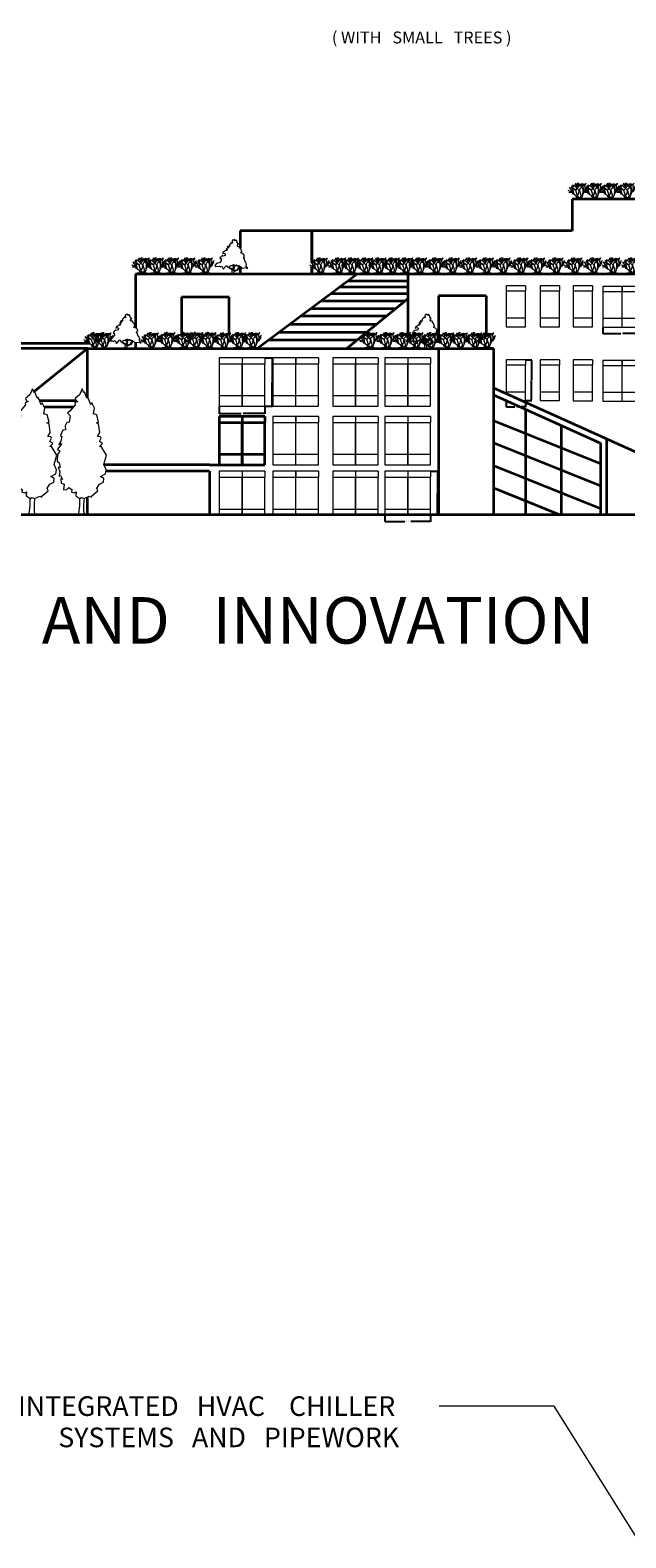
# Model space of a CAD drawing. Units: inches. Extents: x -1080 to 1950, y -1929 to 857.
# Tile 4 of 16: x -30 to 294, y -547 to 272. Entities that reach past the tile are written whole.
import ezdxf

# ---------------------------------------------------------------- set-up
doc = ezdxf.new("R2010")
doc.units = ezdxf.units.IN
doc.header["$MEASUREMENT"] = 0
for name, color, linetype, lineweight in [('A-ANNO-DIMS', 2, 'Continuous', 18), ('A-ANNO-SYMB', 2, 'Continuous', 18), ('A-ANNO-TEXT', 7, 'Continuous', 25), ('A-ELEV', 7, 'Continuous', 35), ('A-GLAZ', 4, 'Continuous', 18), ('L-PLNT', 82, 'Continuous', 13)]:
    doc.layers.add(name, color=color, linetype=linetype, lineweight=lineweight)
doc.styles.get("Standard").update_dxf_attribs({"font": 'arial.ttf'})
doc.dimstyles.get("Standard").update_dxf_attribs({"dimtxt": 0.18, "dimasz": 0.18, "dimexe": 0.18, "dimexo": 0.0625, "dimgap": 0.09, "dimtad": 0, "dimtih": 1, "dimtoh": 1, "dimdec": 4, "dimzin": 0, "dimdsep": 46, "dimtxsty": 'Standard', "dimcen": 0.09, "dimadec": 0, "dimazin": 0, "dimtfac": 1, "dimtdec": 4, "dimtofl": 0, "dimtmove": 0, "dimatfit": 3, "dimfxl": 1, "dimtolj": 1, "dimtzin": 0, "dimarcsym": 0})

# ---------------------------------------------------------------- blocks, each defined once
blk = doc.blocks.new('*U2')
for points in [[(22.0124, 137.721), (18.5475, 141.5624), (15.5282, 138.2446), (13.8028, 139.3505), (13.3714, 142.1153), (11.2148, 143.2214), (8.1954, 140.4564), (4.7447, 141.0094), (2.1567, 136.0326), (2.1567, 131.6088), (5.6074, 129.9499), (3.0193, 128.2909), (0.4313, 130.5029), (-6.9015, 123.3141), (-6.9015, 121.6552), (-9.9208, 119.9963), (-9.0581, 118.3373), (-6.9015, 115.0195), (-10.7835, 112.2546), (-14.6656, 115.0195), (-16.8222, 114.4665), (-17.6849, 112.2546), (-14.6656, 111.7016), (-14.2342, 107.2778), (-17.6065, 107.8307), (-21.5669, 103.9599), (-17.2536, 103.4069), (-18.9789, 97.8771), (-22.8609, 97.3241), (-27.1743, 94.5593), (-32.3504, 91.7944), (-32.7817, 94.0063), (-36.6638, 85.7116), (-29.7624, 87.3705), (-25.449, 84.6056), (-26.743, 77.9699), (-34.507, 75.205), (-37.9578, 77.4169), (-39.2518, 74.099), (-42.2711, 73.5461), (-44.8592, 70.2282), (-47.8786, 66.3574), (-43.9965, 63.0395), (-41.4085, 64.6985), (-44.3346, 59.8898), (-42.2089, 60.1377), (-42.5159, 55.7849), (-49.6039, 46.4502), (-58.2307, 45.8972), (-62.1127, 43.6853), (-68.5828, 36.4966), (-65.9947, 32.0727), (-50.0352, 32.6257), (-47.0159, 30.4138), (-39.6831, 33.7317), (-34.507, 22.6721), (-32.3504, 22.6721), (-22.4296, 34.8376), (-19.4102, 36.4966), (-17.2536, 33.7317), (-17.2536, 29.8608), (-13.8028, 28.7549), (-9.0581, 28.7549), (-7.3328, 32.6257), (-1.7254, 35.3906), (3.8821, 35.9436), (6.4701, 38.1555), (6.9014, 38.7085), (8.1954, 41.4734), (9.9208, 40.3674), (11.2148, 35.9436), (14.2341, 37.6025), (15.0968, 36.4966), (15.9595, 33.7317), (18.9789, 38.7085), (21.9982, 38.7085), (23.2922, 36.4966), (21.9982, 34.2847), (25.4489, 35.3906), (26.743, 33.7317), (29.7623, 35.9436), (32.7817, 34.8376), (38.8204, 28.7549), (41.4084, 27.6489), (43.5651, 25.437), (61.6813, 27.0959), (65.132, 23.7781), (67.7201, 24.884), (60.8186, 33.7317), (60.3873, 37.0495), (62.544, 40.3674), (58.662, 50.874), (56.5053, 50.874), (52.1919, 66.3574), (47.8785, 66.9103), (50.4665, 69.1222), (53.9172, 77.9699), (47.0158, 85.1586), (38.3891, 87.9235), (42.2711, 94.0063)], [(42.2711, 94.0063), (38.8204, 104.5129), (36.6637, 104.5129), (32.3503, 113.9135), (29.7623, 113.3605), (26.743, 113.3605), (24.5862, 117.7844), (25.8802, 123.8671), (29.331, 123.8671), (22.8609, 131.6088), (21.9982, 137.6916)], [(-12.9401, 28.7549), (-2.588, 22.1191), (0.8626, 17.6953), (1.7253, 11.6125), (0, 0)], [(-9.9208, 28.2019), (0, 23.2251), (3.4507, 19.9072), (4.7447, 15.4834), (8.6267, 27.0959), (6.4701, 37.6025)], [(34.5071, 33.1787), (27.1743, 18.2483), (9.0581, 10.5066), (7.7641, 3.8708), (8.1954, 0)], [(8.1954, 40.3674), (11.2148, 27.6489), (8.1954, 13.8245), (24.5862, 19.9072), (32.7817, 34.2847)]]:
    blk.add_lwpolyline(points)
blk = doc.blocks.new('*U5')
blk.add_lwpolyline([(-2.754, 191.699), (-6.78, 182.851), (-13.682, 176.953), (-11.956, 173.266), (-9.656, 172.529), (-14.257, 170.317), (-13.682, 167.368), (-21.733, 157.783), (-25.184, 154.834), (-21.158, 150.41), (-21.733, 147.461), (-22.884, 140.825), (-26.334, 140.087), (-29.21, 134.926), (-28.635, 129.028), (-32.661, 128.291), (-36.111, 120.18), (-34.386, 118.706), (-35.536, 111.333), (-38.987, 106.171), (-34.386, 107.646), (-40.712, 98.798), (-37.261, 95.849), (-40.712, 90.688), (-41.287, 80.366), (-38.412, 78.154), (-36.686, 70.781), (-39.562, 71.518), (-37.261, 64.145), (-38.412, 57.509), (-36.111, 58.247), (-33.236, 52.348), (-35.536, 53.086), (-34.961, 46.45), (-30.36, 44.975), (-31.51, 36.128), (-26.334, 36.865), (-23.459, 39.814), (-18.283, 36.128), (-20.008, 33.178), (-14.832, 31.704), (-11.956, 33.178), (-12.531, 27.28), (-6.205, 22.856), (-3.905, 24.331), (0.121, 22.856), (8.173, 26.543), (11.624, 25.068), (12.199, 27.28), (21.4, 34.653), (19.675, 39.077), (23.701, 44.975), (30.027, 47.924), (30.602, 53.823), (25.426, 56.772), (32.903, 61.196), (34.053, 67.094), (30.602, 75.205), (34.628, 89.951), (26.576, 103.222), (23.701, 103.222), (28.302, 107.646), (23.701, 110.595), (26.576, 115.756), (25.426, 117.968), (20.825, 118.706), (24.276, 124.604), (22.551, 137.876), (19.1, 139.35), (22.551, 140.825), (19.675, 151.884), (14.499, 153.359), (16.224, 162.207), (12.199, 170.317), (10.473, 167.368), (5.872, 179.165), (4.147, 177.69), (0.696, 187.275), (-0.454, 185.8)], close=True)
for points in [[(-6.813, 23.669), (-6.813, 11.669), (-8.627, 0)], [(0.387, 23.669), (-0.576, 13.271), (-0.576, 3.686), (0, 0)]]:
    blk.add_lwpolyline(points)
blk = doc.blocks.new('*U6')
for p, q in [((-316.7634, 502.285), (-327.6092, 559.9176)), ((-290.3982, 464.5406), (-265.6078, 577.8246)), ((-207.264, 451.104), (-268.224, 548.64)), ((-240.792, 502.285), (-228.3968, 573.8368)), ((-129.1844, 450.6214), (-140.0302, 542.036)), ((-134.112, 487.68), (-97.536, 548.64)), ((-85.7758, 472.4908), (-73.3552, 548.005)), ((-12.9032, 555.9552), (-2.0574, 522.1732)), ((-5.1562, 486.3846), (2.5908, 542.036)), ((1.0414, 526.1356), (35.1536, 559.9176)), ((2.5908, 542.036), (21.209, 555.9552)), ((-451.104, 219.456), (-601.0402, 303.8094)), ((-451.104, 219.456), (-587.4512, 234.2388)), ((-463.296, 280.416), (-552.577, 423.037)), ((-463.296, 280.416), (-512.064, 292.608)), ((-329.184, 316.992), (-499.872, 414.528)), ((-353.568, 316.992), (-487.68, 377.952)), ((-426.72, 414.528), (-475.488, 475.488)), ((-402.336, 207.264), (-463.296, 280.416)), ((-414.528, 182.88), (-463.296, 182.88)), ((-377.952, 463.296), (-451.104, 487.68)), ((-426.72, 316.992), (-451.104, 329.184)), ((-377.952, 146.304), (-451.104, 219.456)), ((-402.336, 12.192), (-451.104, 0)), ((-426.72, 414.528), (-390.144, 499.872)), ((-426.72, 316.992), (-426.72, 414.528)), ((-402.336, 207.264), (-426.72, 316.992)), ((-377.952, 146.304), (-402.336, 207.264)), ((-341.376, 12.192), (-402.336, 12.192)), ((-377.952, 463.296), (-329.184, 524.256)), ((-207.264, 304.8), (-377.952, 463.296)), ((-329.184, 121.92), (-377.952, 146.304)), ((-329.184, 316.992), (-353.568, 316.992)), ((-243.84, 24.384), (-341.376, 12.192)), ((-338.455, 424.7896), (-290.3982, 464.5406)), ((-329.184, 316.992), (-207.264, 451.104)), ((-268.224, 109.728), (-329.184, 316.992)), ((-292.608, 60.96), (-329.184, 121.92)), ((-243.84, 24.384), (-329.184, 0)), ((-296.5958, 484.4034), (-316.7634, 502.285)), ((-286.512, 498.3226), (-307.4416, 538.0736)), ((-305.8922, 396.9512), (-302.7934, 478.4344)), ((-304.3428, 426.7708), (-268.7066, 458.5716)), ((-302.7934, 478.4344), (-270.256, 518.1854)), ((-219.456, 24.384), (-292.608, 60.96)), ((-268.7066, 458.5716), (-250.0884, 500.3038)), ((-268.224, 109.728), (-219.456, 195.072)), ((-219.456, 48.768), (-268.224, 109.728)), ((-243.84, 24.384), (-195.072, 24.384)), ((-182.88, 499.872), (-219.456, 512.064)), ((-219.456, 195.072), (-207.264, 304.8)), ((-219.456, 24.384), (-109.728, 73.152)), ((-219.456, 24.384), (-158.496, 73.152)), ((-219.456, 24.384), (-219.456, 48.768)), ((-219.456, 24.384), (-73.152, 24.384)), ((-207.264, 451.104), (-134.112, 487.68)), ((-195.072, 316.992), (-182.88, 377.952)), ((-170.688, 219.456), (-195.072, 316.992)), ((-195.072, 24.384), (-158.496, 12.192)), ((-182.88, 499.872), (-158.496, 536.448)), ((-121.92, 414.528), (-182.88, 499.872)), ((-182.88, 377.952), (-97.536, 426.72)), ((-146.304, 134.112), (-170.688, 219.456)), ((-158.496, 73.152), (-146.304, 134.112)), ((-158.496, 12.192), (-85.344, 0)), ((-85.7758, 389.001), (-129.1844, 452.6026)), ((-73.152, 329.184), (-109.728, 499.872)), ((-109.728, 73.152), (-48.768, 243.84)), ((-97.536, 426.72), (-24.384, 524.256)), ((-70.2564, 426.7708), (-85.7758, 472.4908)), ((-85.344, 134.112), (-73.152, 329.184)), ((-73.152, 402.336), (-60.96, 512.064)), ((-24.384, 268.224), (-73.152, 402.336)), ((-73.152, 24.384), (0, 0)), ((-48.768, 243.84), (24.384, 304.8)), ((-12.192, 274.32), (8.7884, 335.3562)), ((8.7884, 335.3562), (-5.1562, 486.3846)), ((-3.6068, 492.3536), (14.986, 518.1854)), ((-0.508, 508.254), (22.7584, 536.067)), ((8.7884, 335.3562), (33.6042, 412.8516)), ((24.384, 304.8), (36.576, 390.144)), ((24.384, 304.8), (73.152, 377.952)), ((33.6042, 412.8516), (92.5068, 464.5406)), ((36.576, 390.144), (73.152, 438.912)), ((48.768, 341.376), (60.96, 390.144)), ((60.96, 390.144), (85.344, 414.528))]:
    blk.add_line(p, q)
blk = doc.blocks.new('WIN-TYPE-A')
for p, q in [((12.45, 26.32), (0, 26.32)), ((0, 26.32), (0, 23.06)), ((24.78, 26.32), (12.34, 26.32)), ((12.34, 26.32), (12.34, 23.06)), ((12.45, 26.32), (12.45, 23.06)), ((24.78, 26.32), (24.78, 23.06)), ((0, 23.06), (0, 5.73)), ((0, 23.06), (12.45, 23.06)), ((12.34, 23.06), (12.34, 5.73)), ((12.34, 23.06), (24.78, 23.06)), ((12.45, 5.73), (12.45, 23.06)), ((24.78, 5.73), (24.78, 23.06)), ((0, 5.73), (12.45, 5.73)), ((0, 5.73), (0, 0)), ((0, 0), (12.45, 0)), ((12.34, 5.73), (24.78, 5.73)), ((12.34, 5.73), (12.34, 0)), ((12.34, 0), (24.78, 0)), ((12.45, 0), (12.45, 5.73)), ((24.78, 0), (24.78, 5.73))]:
    blk.add_line(p, q)
blk = doc.blocks.new('WIN-TYPE-B')
for p, q in [((10.5, 22.21), (0, 22.21)), ((0, 22.21), (0, 19.45)), ((0, 19.45), (0, 4.84)), ((0, 19.45), (10.5, 19.45)), ((20.91, 22.21), (10.41, 22.21)), ((10.41, 22.21), (10.41, 19.45)), ((10.41, 19.45), (10.41, 4.84)), ((10.41, 19.45), (20.91, 19.45)), ((10.5, 22.21), (10.5, 19.45)), ((10.5, 4.84), (10.5, 19.45)), ((20.91, 22.21), (20.91, 19.45)), ((20.91, 4.84), (20.91, 19.45)), ((0, 4.84), (10.5, 4.84)), ((0, 4.84), (0, 0)), ((0, 0), (10.5, 0)), ((10.41, 4.84), (20.91, 4.84)), ((10.41, 4.84), (10.41, 0)), ((10.41, 0), (20.91, 0)), ((10.5, 0), (10.5, 4.84)), ((20.91, 0), (20.91, 4.84))]:
    blk.add_line(p, q)
blk = doc.blocks.new('WIN-TYPE-C')
for p, q in [((12.45, 23.64), (0, 23.64)), ((0, 23.64), (0, 20.37)), ((0, 20.37), (0, 3.04)), ((0, 20.37), (12.45, 20.37)), ((24.78, 23.64), (12.34, 23.64)), ((12.34, 23.64), (12.34, 20.37)), ((12.34, 20.37), (12.34, 3.04)), ((12.34, 20.37), (24.78, 20.37)), ((12.45, 23.64), (12.45, 20.37)), ((12.45, 3.04), (12.45, 20.37)), ((24.78, 23.64), (24.78, 20.37)), ((24.78, 3.04), (24.78, 20.37)), ((0, 3.04), (12.45, 3.04)), ((0, 3.04), (0, 0)), ((12.34, 3.04), (24.78, 3.04)), ((12.34, 3.04), (12.34, 0)), ((12.45, 0), (12.45, 3.04)), ((24.78, 0), (24.78, 3.04))]:
    blk.add_line(p, q)
blk = doc.blocks.new('WIN-TYPE-E')
for p, q in [((10.5, 22.21), (0, 22.21)), ((0, 22.21), (0, 19.45)), ((0, 19.45), (0, 4.84)), ((0, 19.45), (10.5, 19.45)), ((10.5, 22.21), (10.5, 19.45)), ((10.5, 4.84), (10.5, 19.45)), ((0, 4.84), (10.5, 4.84)), ((0, 4.84), (0, 0)), ((0, 0), (10.5, 0)), ((10.5, 0), (10.5, 4.84))]:
    blk.add_line(p, q)
blk = doc.blocks.new('WIN-TYPE-P')
for p, q in [((10.5, 22.21), (0, 22.21)), ((0, 22.21), (0, 19.45)), ((0, 19.45), (0, 4.84)), ((0, 19.45), (10.5, 19.45)), ((10.5, 22.21), (10.5, 19.45)), ((10.5, 4.84), (10.5, 19.45)), ((0, 4.84), (10.5, 4.84)), ((0, 4.84), (0, 3.89)), ((8.62, 0), (10.5, 0)), ((10.5, 0), (10.5, 4.84))]:
    blk.add_line(p, q)
blk = doc.blocks.new('*D35')
at = {"layer": 'A-ANNO-DIMS', "color": 0, "lineweight": -2, "transparency": 16777216}
for p, q in [((97.82, 94.4), (101.89, 94.4)), ((101.71, 94.22), (101.71, 81.42)), ((101.71, 68.26), (101.71, 81.06)), ((97.82, 68.08), (101.89, 68.08))]:
    blk.add_line(p, q, dxfattribs=at)
at = {"layer": 'A-ANNO-DIMS', "color": 0, "transparency": 16777216}
for points in [[(101.68, 94.22), (101.74, 94.22), (101.71, 94.4)], [(101.68, 68.26), (101.74, 68.26), (101.71, 68.08)]]:
    blk.add_solid(points, dxfattribs=at)
at = {"layer": 'Defpoints', "color": 0, "transparency": 16777216}
for p in [(97.76, 94.4), (101.71, 94.4), (97.76, 68.08)]:
    blk.add_point(p, dxfattribs=at)
at = {"layer": 'A-ANNO-DIMS', "color": 0, "transparency": 16777216, "insert": (101.71, 81.24), "char_height": 0.18, "attachment_point": 5}
blk.add_mtext('\\A1;WINDOW TYPE A 26 TYP.', dxfattribs=at)
blk = doc.blocks.new('*D36')
at = {"layer": 'A-ANNO-DIMS', "color": 0, "lineweight": -2, "transparency": 16777216}
for p, q in [((72.97, 68.01), (72.97, 63.95)), ((97.76, 68.01), (97.76, 63.95)), ((73.15, 64.13), (84.83, 64.13)), ((97.58, 64.13), (85.89, 64.13))]:
    blk.add_line(p, q, dxfattribs=at)
at = {"layer": 'A-ANNO-DIMS', "color": 0, "transparency": 16777216}
for points in [[(73.15, 64.16), (73.15, 64.1), (72.97, 64.13)], [(97.58, 64.16), (97.58, 64.1), (97.76, 64.13)]]:
    blk.add_solid(points, dxfattribs=at)
at = {"layer": 'Defpoints', "color": 0, "transparency": 16777216}
for p in [(72.97, 68.08), (97.76, 68.08), (97.76, 64.13)]:
    blk.add_point(p, dxfattribs=at)
at = {"layer": 'A-ANNO-DIMS', "color": 0, "transparency": 16777216, "insert": (85.36, 64.13), "char_height": 0.18, "attachment_point": 5}
blk.add_mtext('\\A1;25 TYP.', dxfattribs=at)
blk = doc.blocks.new('*D38')
at = {"layer": 'A-ANNO-DIMS', "color": 0, "lineweight": -2, "transparency": 16777216}
for p, q in [((281.34, 110.89), (281.34, 107.44)), ((281.52, 107.62), (291.27, 107.62)), ((302.07, 107.62), (292.33, 107.62)), ((302.25, 110.89), (302.25, 107.44))]:
    blk.add_line(p, q, dxfattribs=at)
at = {"layer": 'A-ANNO-DIMS', "color": 0, "transparency": 16777216}
for points in [[(281.52, 107.65), (281.52, 107.59), (281.34, 107.62)], [(302.07, 107.65), (302.07, 107.59), (302.25, 107.62)]]:
    blk.add_solid(points, dxfattribs=at)
at = {"layer": 'Defpoints', "color": 0, "transparency": 16777216}
for p in [(281.34, 110.95), (302.25, 110.95), (302.25, 107.62)]:
    blk.add_point(p, dxfattribs=at)
at = {"layer": 'A-ANNO-DIMS', "color": 0, "transparency": 16777216, "insert": (291.8, 107.62), "char_height": 0.18, "attachment_point": 5}
blk.add_mtext('\\A1;21 TYP.', dxfattribs=at)
blk = doc.blocks.new('*D39')
at = {"layer": 'A-ANNO-DIMS', "color": 0, "lineweight": -2, "transparency": 16777216}
for p, q in [((163.01, 8.96), (163.01, 5.12)), ((187.79, 8.96), (187.79, 5.12)), ((163.19, 5.3), (173.79, 5.3)), ((187.61, 5.3), (177.01, 5.3))]:
    blk.add_line(p, q, dxfattribs=at)
at = {"layer": 'A-ANNO-DIMS', "color": 0, "transparency": 16777216}
for points in [[(163.19, 5.33), (163.19, 5.27), (163.01, 5.3)], [(187.61, 5.33), (187.61, 5.27), (187.79, 5.3)]]:
    blk.add_solid(points, dxfattribs=at)
at = {"layer": 'Defpoints', "color": 0, "transparency": 16777216}
for p in [(163.01, 9.02), (187.79, 9.02), (187.79, 5.3)]:
    blk.add_point(p, dxfattribs=at)
at = {"layer": 'A-ANNO-DIMS', "color": 0, "transparency": 16777216, "insert": (175.4, 5.3), "char_height": 0.18, "attachment_point": 5}
blk.add_mtext('\\A1;WINDOW TYPE C 25 TYP.', dxfattribs=at)
blk = doc.blocks.new('*D40')
at = {"layer": 'A-ANNO-DIMS', "color": 0, "lineweight": -2, "transparency": 16777216}
for p, q in [((187.85, 32.66), (191.69, 32.66)), ((191.51, 32.48), (191.51, 21.02)), ((191.51, 9.2), (191.51, 20.66)), ((187.85, 9.02), (191.69, 9.02))]:
    blk.add_line(p, q, dxfattribs=at)
at = {"layer": 'A-ANNO-DIMS', "color": 0, "transparency": 16777216}
for points in [[(191.48, 32.48), (191.54, 32.48), (191.51, 32.66)], [(191.48, 9.2), (191.54, 9.2), (191.51, 9.02)]]:
    blk.add_solid(points, dxfattribs=at)
at = {"layer": 'Defpoints', "color": 0, "transparency": 16777216}
for p in [(187.79, 32.66), (191.51, 32.66), (187.79, 9.02)]:
    blk.add_point(p, dxfattribs=at)
at = {"layer": 'A-ANNO-DIMS', "color": 0, "transparency": 16777216, "insert": (191.51, 20.84), "char_height": 0.18, "attachment_point": 5}
blk.add_mtext('\\A1;24 TYP.', dxfattribs=at)
blk = doc.blocks.new('*D61')
at = {"layer": 'A-ANNO-DIMS', "color": 0, "lineweight": -2, "transparency": 16777216}
for p, q in [((239.38, 93.27), (242.83, 93.27)), ((242.65, 93.09), (242.65, 82.35)), ((242.65, 71.24), (242.65, 81.99)), ((239.38, 71.06), (242.83, 71.06))]:
    blk.add_line(p, q, dxfattribs=at)
at = {"layer": 'A-ANNO-DIMS', "color": 0, "transparency": 16777216}
for points in [[(242.62, 93.09), (242.68, 93.09), (242.65, 93.27)], [(242.62, 71.24), (242.68, 71.24), (242.65, 71.06)]]:
    blk.add_solid(points, dxfattribs=at)
at = {"layer": 'Defpoints', "color": 0, "transparency": 16777216}
for p in [(239.32, 93.27), (242.65, 93.27), (239.32, 71.06)]:
    blk.add_point(p, dxfattribs=at)
at = {"layer": 'A-ANNO-DIMS', "color": 0, "transparency": 16777216, "insert": (242.65, 82.17), "char_height": 0.18, "attachment_point": 5}
blk.add_mtext('\\A1;WINDOW TYPE P 22 TYP.', dxfattribs=at)
blk = doc.blocks.new('*D62')
at = {"layer": 'A-ANNO-DIMS', "color": 0, "lineweight": -2, "transparency": 16777216}
for p, q in [((228.82, 71), (228.82, 67.55)), ((229, 67.73), (233.55, 67.73)), ((239.14, 67.73), (234.59, 67.73)), ((239.32, 71), (239.32, 67.55))]:
    blk.add_line(p, q, dxfattribs=at)
at = {"layer": 'A-ANNO-DIMS', "color": 0, "transparency": 16777216}
for points in [[(229, 67.76), (229, 67.7), (228.82, 67.73)], [(239.14, 67.76), (239.14, 67.7), (239.32, 67.73)]]:
    blk.add_solid(points, dxfattribs=at)
at = {"layer": 'Defpoints', "color": 0, "transparency": 16777216}
for p in [(228.82, 71.06), (239.32, 71.06), (239.32, 67.73)]:
    blk.add_point(p, dxfattribs=at)
at = {"layer": 'A-ANNO-DIMS', "color": 0, "transparency": 16777216, "insert": (234.07, 67.73), "char_height": 0.18, "attachment_point": 5}
blk.add_mtext('\\A1;11 TYP.', dxfattribs=at)

msp = doc.modelspace()

# ---------------------------------------------------------------- linework, layer by layer
at = {"layer": 'A-ANNO-SYMB'}
for p, q in [((254.91, -475.48), (192.41, -475.48)), ((299.91, -546.98), (254.91, -475.48))]:
    msp.add_line(p, q, dxfattribs=at)
at = {"layer": 'A-ELEV'}
for p, q in [((264.78, 180.63), (264.78, 163.4)), ((445.1, 180.63), (264.78, 180.63)), ((84.25, 163.4), (84.25, 153.85)), ((123.28, 163.4), (84.25, 163.4)), ((264.78, 163.4), (121.84, 163.4)), ((123.28, 163.4), (123.28, 145.94)), ((123.28, 145.94), (123.28, 163.4)), ((311.23, 139.7), (27.33, 139.7)), ((27.33, 139.7), (27.33, 110.56)), ((84.25, 143.98), (84.25, 139.7)), ((84.25, 142.55), (84.25, 140.7)), ((147.93, 139.7), (93.65, 99.4)), ((123.28, 143.57), (123.28, 139.7)), ((123.28, 139.7), (123.28, 143.57)), ((175.64, 104.8), (175.64, 139.7)), ((138.87, 132.98), (175.64, 132.98)), ((143.17, 136.17), (175.64, 136.17)), ((78.3, 127.31), (52.42, 127.31)), ((52.42, 127.31), (52.42, 107.83)), ((78.3, 107.26), (78.3, 127.31)), ((128.53, 125.3), (174.06, 125.3)), ((133.94, 129.31), (175.64, 129.31)), ((175.64, 126.59), (142.33, 99.4)), ((217.97, 127.96), (192.09, 127.96)), ((192.09, 127.96), (192.09, 105.94)), ((217.97, 127.96), (217.97, 105.75)), ((117.54, 117.14), (164.06, 117.14)), ((122.91, 121.13), (168.95, 121.13)), ((105.48, 108.19), (153.09, 108.19)), ((111.45, 112.62), (158.52, 112.62)), ((1.28, 99.4), (-126.4, 99.4)), ((-123.32, 102.28), (2.16, 102.28)), ((1.28, 99.4), (-27.9, 75.82)), ((1.28, 72.79), (1.28, 99.4)), ((1.28, 99.4), (221.43, 99.4)), ((27.33, 102.6), (27.33, 99.4)), ((52.42, 106.21), (52.42, 105.86)), ((52.42, 104.47), (52.42, 104.15)), ((78.3, 103.03), (78.3, 103.83)), ((78.3, 99.4), (78.3, 99.5)), ((99.98, 104.1), (148.09, 104.1)), ((175.64, 99.4), (175.64, 99.82)), ((192.09, 99.4), (192.09, 9.02)), ((221.9, 99.4), (213.13, 99.4)), ((217.97, 100.02), (217.97, 99.85)), ((221.9, 99.4), (221.43, 99.4)), ((221.9, 99.4), (221.9, 9.02)), ((221.9, 78.07), (374.96, 9.02)), ((221.9, 74.27), (280.06, 47.95)), ((-4.84, 70.95), (-24.69, 70.95)), ((-6.46, 67.56), (-22.1, 67.56)), ((239.32, 66.39), (239.32, 9.02)), ((85.42, 62.51), (72.97, 62.51)), ((72.97, 62.51), (72.97, 59.24)), ((72.97, 59.24), (72.97, 41.92)), ((72.97, 59.24), (85.42, 59.24)), ((97.76, 62.51), (85.31, 62.51)), ((85.31, 62.51), (85.31, 59.24)), ((85.31, 59.24), (85.31, 41.92)), ((85.31, 59.24), (97.76, 59.24)), ((85.42, 62.51), (85.42, 59.24)), ((85.42, 41.92), (85.42, 59.24)), ((97.76, 62.51), (97.76, 59.24)), ((97.76, 41.92), (97.76, 59.24)), ((221.9, 60.25), (280.06, 36.88)), ((258.81, 57.57), (258.81, 9.02)), ((280.06, 51.98), (280.06, 51.84)), ((283.36, 50.35), (283.36, 9.02)), ((72.97, 41.92), (85.42, 41.92)), ((72.97, 41.92), (72.97, 36.18)), ((85.31, 41.92), (97.76, 41.92)), ((85.31, 41.92), (85.31, 36.18)), ((85.42, 36.18), (85.42, 41.92)), ((97.76, 36.18), (97.76, 41.92)), ((221.86, 48.23), (280.02, 24.86)), ((280.06, 47.95), (280.06, 9.02)), ((67.63, 36.18), (10.26, 36.18)), ((67.63, 36.18), (72.97, 36.18)), ((72.97, 36.18), (85.42, 36.18)), ((85.31, 36.18), (97.76, 36.18)), ((221.54, 36), (279.69, 12.63)), ((67.63, 32.66), (11.28, 32.66)), ((67.63, 32.66), (67.63, 9.02)), ((1.28, 9.02), (1.28, 18.65)), ((221.9, 23.63), (258.25, 9.02)), ((709.45, 9.02), (-148.56, 9.02))]:
    msp.add_line(p, q, dxfattribs=at)

# ---------------------------------------------------------------- block references
at = {"layer": 'A-GLAZ'}
for name, p in [('WIN-TYPE-E', (228.82, 111.23)), ('WIN-TYPE-E', (247.31, 111.23)), ('WIN-TYPE-E', (265.26, 111.23)), ('WIN-TYPE-B', (281.34, 110.95)), ('WIN-TYPE-A', (72.97, 68.08)), ('WIN-TYPE-A', (102.08, 68.08)), ('WIN-TYPE-A', (134.59, 68.08)), ('WIN-TYPE-A', (163.01, 68.08)), ('WIN-TYPE-P', (228.82, 71.06)), ('WIN-TYPE-E', (247.31, 71.06)), ('WIN-TYPE-E', (265.26, 71.02)), ('WIN-TYPE-B', (281.34, 70.74)), ('WIN-TYPE-A', (102.08, 36.18)), ('WIN-TYPE-A', (134.59, 36.18)), ('WIN-TYPE-A', (163.01, 36.18)), ('WIN-TYPE-C', (72.97, 9.02)), ('WIN-TYPE-C', (102.08, 9.02)), ('WIN-TYPE-C', (134.59, 9.02)), ('WIN-TYPE-C', (163.01, 9.02))]:
    msp.add_blockref(name, p, dxfattribs=at)
at = {"layer": 'L-PLNT'}
for name, p, xscale, yscale, zscale in [('*U6', (271.79, 180.68), 0.0152219259934872, 0.0152219259934872, 0.0152219259934872), ('*U6', (280.19, 180.68), 0.0152219259934872, 0.0152219259934872, 0.0152219259934872), ('*U6', (288.96, 180.68), 0.0152219259934872, 0.0152219259934872, 0.0152219259934872), ('*U6', (297.89, 180.68), 0.0152219259934872, 0.0152219259934872, 0.0152219259934872), ('*U2', (79.58, 139.76), 0.1315554675521508, 0.1315554675521508, 0.1315554675521508), ('*U6', (34.48, 140.11), 0.0152219259934872, 0.0152219259934872, 0.0152219259934872), ('*U6', (42.13, 140.11), 0.0152219259934872, 0.0152219259934872, 0.0152219259934872), ('*U6', (50.37, 140.11), 0.0152219259934872, 0.0152219259934872, 0.0152219259934872), ('*U6', (59.22, 140.11), 0.0152219259934872, 0.0152219259934872, 0.0152219259934872), ('*U6', (68.7, 140.11), 0.0152219259934872, 0.0152219259934872, 0.0152219259934872), ('*U6', (131.31, 140.11), 0.0152219259934872, 0.0152219259934872, 0.0152219259934872), ('*U6', (141.23, 140.11), 0.0152219259934872, 0.0152219259934872, 0.0152219259934872), ('*U6', (148.34, 140.11), 0.0152219259934872, 0.0152219259934872, 0.0152219259934872), ('*U6', (155.88, 140.11), 0.0152219259934872, 0.0152219259934872, 0.0152219259934872), ('*U6', (163.15, 140.11), 0.0152219259934872, 0.0152219259934872, 0.0152219259934872), ('*U6', (170.4, 140.11), 0.0152219259934872, 0.0152219259934872, 0.0152219259934872), ('*U6', (177.65, 140.11), 0.0152219259934872, 0.0152219259934872, 0.0152219259934872), ('*U6', (185.17, 140.11), 0.0152219259934872, 0.0152219259934872, 0.0152219259934872), ('*U6', (194.04, 140.11), 0.0152219259934872, 0.0152219259934872, 0.0152219259934872), ('*U6', (203.06, 140.11), 0.0152219259934872, 0.0152219259934872, 0.0152219259934872), ('*U6', (212.38, 140.11), 0.0152219259934872, 0.0152219259934872, 0.0152219259934872), ('*U6', (221.49, 140.11), 0.0152219259934872, 0.0152219259934872, 0.0152219259934872), ('*U6', (230.57, 140.11), 0.0152219259934872, 0.0152219259934872, 0.0152219259934872), ('*U6', (240.21, 140.11), 0.0152219259934872, 0.0152219259934872, 0.0152219259934872), ('*U6', (249.29, 140.11), 0.0152219259934872, 0.0152219259934872, 0.0152219259934872), ('*U6', (259.37, 140.11), 0.0152219259934872, 0.0152219259934872, 0.0152219259934872), ('*U6', (269.58, 140.11), 0.0152219259934872, 0.0152219259934872, 0.0152219259934872), ('*U6', (279.8, 140.11), 0.0152219259934872, 0.0152219259934872, 0.0152219259934872), ('*U6', (290.15, 140.11), 0.0152219259934872, 0.0152219259934872, 0.0152219259934872), ('*U6', (300.62, 140.11), 0.0152219259934872, 0.0152219259934872, 0.0152219259934872), ('*U2', (21.5, 99.24), 0.1315554675521508, 0.1315554675521508, 0.1315554675521508), ('*U2', (184.32, 99.24), 0.1315554675521508, 0.1315554675521508, 0.1315554675521508), ('*U6', (8.49, 99.47), 0.0152219259934872, 0.0152219259934872, 0.0152219259934872), ('*U6', (13.73, 99.47), 0.0152219259934872, 0.0152219259934872, 0.0152219259934872), ('*U6', (39.38, 99.47), 0.0152219259934872, 0.0152219259934872, 0.0152219259934872), ('*U6', (48.37, 99.57), 0.0152219259934872, 0.0152219259934872, 0.0152219259934872), ('*U6', (57.36, 99.57), 0.0152219259934872, 0.0152219259934872, 0.0152219259934872), ('*U6', (63.64, 99.57), 0.0152219259934872, 0.0152219259934872, 0.0152219259934872), ('*U6', (70.72, 99.57), 0.0152219259934872, 0.0152219259934872, 0.0152219259934872), ('*U6', (78.73, 99.35), 0.0152219259934872, 0.0152219259934872, 0.0152219259934872), ('*U6', (86.93, 99.5), 0.0152219259934872, 0.0152219259934872, 0.0152219259934872), ('*U6', (94.44, 99.5), 0.0152219259934872, 0.0152219259934872, 0.0152219259934872), ('*U6', (158.21, 99.55), 0.0152219259934872, 0.0152219259934872, 0.0152219259934872), ('*U6', (167.51, 99.55), 0.0152219259934872, 0.0152219259934872, 0.0152219259934872), ('*U6', (176.45, 99.55), 0.0152219259934872, 0.0152219259934872, 0.0152219259934872), ('*U6', (183.31, 99.55), 0.0152219259934872, 0.0152219259934872, 0.0152219259934872), ('*U6', (191.36, 99.47), 0.0152219259934872, 0.0152219259934872, 0.0152219259934872), ('*U6', (199.88, 99.47), 0.0152219259934872, 0.0152219259934872, 0.0152219259934872), ('*U6', (207.3, 99.47), 0.0152219259934872, 0.0152219259934872, 0.0152219259934872), ('*U6', (215.18, 99.47), 0.0152219259934872, 0.0152219259934872, 0.0152219259934872), ('*U6', (221.66, 99.47), 0.0152219259934872, 0.0152219259934872, 0.0152219259934872), ('*U5', (-27.54, 9.75), 0.3528399638811642, 0.3528399638811642, 0.3528399638811642), ('*U5', (-0.58, 9.75), 0.3528399638811642, 0.3528399638811642, 0.3528399638811642)]:
    msp.add_blockref(name, p, dxfattribs=dict(at, xscale=xscale, yscale=yscale, zscale=zscale))

# ---------------------------------------------------------------- texts
at = {"layer": 'A-ANNO-TEXT'}
for s, height, p in [('( WITH   SMALL   TREES )', 6.4607, (134.14, 265.19)), ('FRONT   ELEVATION - MAIN   ACADEMIC   AND   INNOVATION   COMPLEX', 25.272, (-665.96, -61.01)), ('INTEGRATED   HVAC    CHILLER', 10.6643, (-36.54, -480.72)), ('SYSTEMS   AND   PIPEWORK ', 10.6643, (-14.54, -497.72))]:
    msp.add_text(s, height=height, dxfattribs=at).set_placement(p)

# ---------------------------------------------------------------- dimensions: what is measured, and where the dimension line sits
at = {"layer": 'A-ANNO-DIMS'}
for base, p1, p2, text, picture, middle in [((302.25, 107.62), (281.34, 110.95), (302.25, 110.95), '<> TYP.', '*D38', (291.8, 107.62)), ((97.76, 64.13), (72.97, 68.08), (97.76, 68.08), '<> TYP.', '*D36', (85.36, 64.13)), ((239.3213, 67.7328), (228.8188, 71.0641), (239.3213, 71.0641), '<> TYP.', '*D62', (234.0701, 67.7328)), ((187.79, 5.3), (163.01, 9.02), (187.79, 9.02), 'WINDOW TYPE C <> TYP.', '*D39', (175.4, 5.3))]:
    dim = msp.add_linear_dim(base=base, p1=p1, p2=p2, text=text, dimstyle='Standard', override={"dimdec": 0, "dimlfac": 1, "dimrnd": 0, "dimzin": 0, "dimdsep": 46, "dimlunit": 2}, dxfattribs=at)
    dim.commit()
    dim.dimension.update_dxf_attribs({"geometry": picture, "text_midpoint": middle})
for base, p1, p2, text, picture, middle in [((101.71, 94.4), (97.76, 68.08), (97.76, 94.4), 'WINDOW TYPE A <> TYP.', '*D35', (101.71, 81.24)), ((242.65, 93.27), (239.32, 71.06), (239.32, 93.27), 'WINDOW TYPE P <> TYP.', '*D61', (242.65, 82.17)), ((191.51, 32.66), (187.79, 9.02), (187.79, 32.66), '<> TYP.', '*D40', (191.51, 20.84))]:
    dim = msp.add_linear_dim(base=base, p1=p1, p2=p2, angle=90, text=text, dimstyle='Standard', override={"dimdec": 0, "dimlfac": 1, "dimrnd": 0, "dimzin": 0, "dimdsep": 46, "dimlunit": 2}, dxfattribs=at)
    dim.commit()
    dim.dimension.update_dxf_attribs({"geometry": picture, "text_midpoint": middle})

doc.saveas('drawing.dxf')
